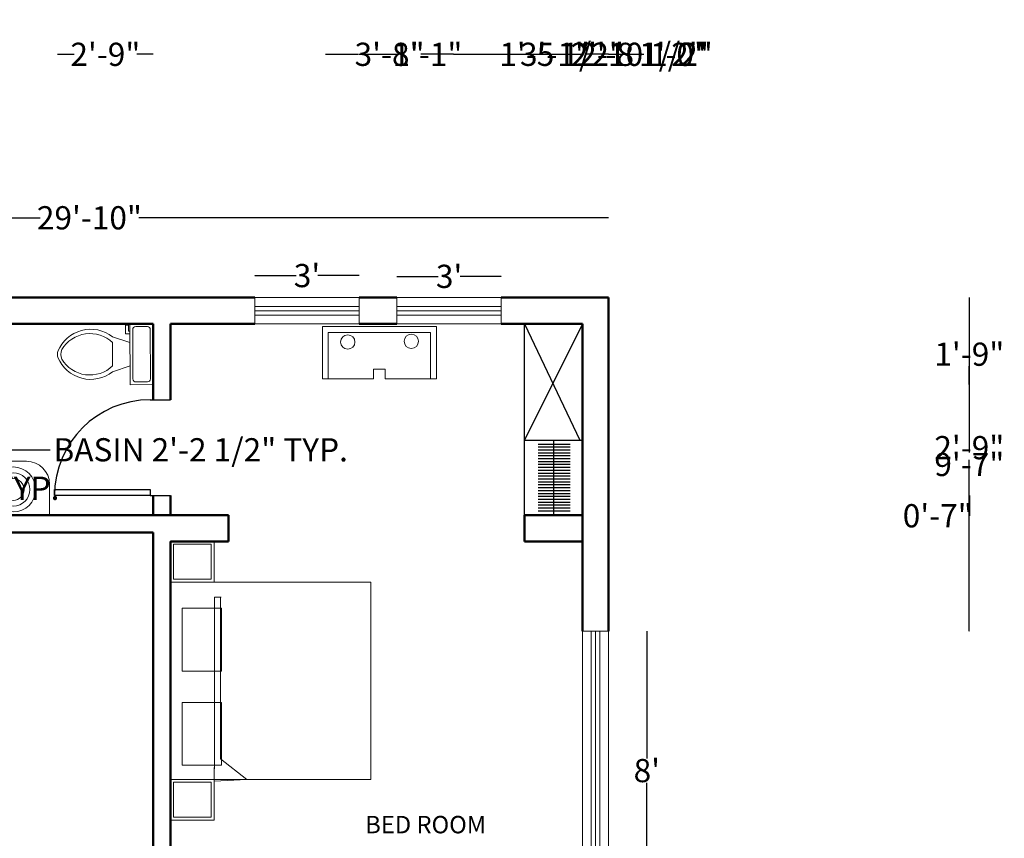
# Model space of a CAD drawing. Units: inches. Extents: x -135167 to -134597, y 156853 to 157819.
# Tile 5 of 5: x -134948 to -134608, y 157537 to 157819. Entities that reach past the tile are written whole.
import ezdxf

# ---------------------------------------------------------------- set-up
doc = ezdxf.new("R2010")
doc.units = ezdxf.units.IN
doc.header["$MEASUREMENT"] = 0
for name, color, linetype, lineweight in [('A-ANNO-DIMS', 4, 'Continuous', 18), ('A-AREA-IDEN', 76, 'Continuous', 25), ('A-FLOR-CASE', 1, 'Continuous', 25), ('A-FLOR-FIXT', 3, 'Continuous', 20), ('A-FURN', 1, 'Continuous', 18), ('doors', 5, 'Continuous', 25), ('walls', 2, 'Continuous', 50), ('window', 6, 'Continuous', 18)]:
    doc.layers.add(name, color=color, linetype=linetype, lineweight=lineweight)
doc.styles.get("Standard").update_dxf_attribs({"font": 'arial.ttf'})
doc.dimstyles.get("Standard").update_dxf_attribs({"dimtxt": 8, "dimasz": 0.18, "dimexe": 0.18, "dimexo": 0.0625, "dimgap": 0.09, "dimtad": 0, "dimtih": 1, "dimtoh": 1, "dimdec": 0, "dimzin": 0, "dimdsep": 46, "dimlunit": 3, "dimtxsty": 'Standard', "dimblk": 'ARCHTICK', "dimcen": 0.09, "dimse1": 1, "dimse2": 1, "dimadec": 0, "dimazin": 0, "dimtfac": 1, "dimtdec": 0, "dimtofl": 0, "dimtmove": 0, "dimatfit": 3, "dimldrblk": 'DOTSMALL', "dimfxl": 1, "dimtolj": 1, "dimtzin": 0, "dimarcsym": 0})

# ---------------------------------------------------------------- blocks, each defined once
blk = doc.blocks.new('*U8')
for p, q in [((0, 0), (0, -6)), ((28, 0), (28, -6))]:
    blk.add_line(p, q)
blk.add_lwpolyline([(0, 0), (0, 28), (1.75, 28), (1.75, 0)], close=True)
blk.add_arc((0, 0), 28, 0, 90)
blk = doc.blocks.new('*U16')
for p, q in [((-9.51, 6.98), (-9.52, 9.98)), ((-9.52, 9.98), (-8.52, 9.98)), ((-8.01, 6.98), (-9.51, 6.98)), ((-8.52, 9.98), (-8.52, 7.98)), ((-8.52, 7.98), (-8.02, 7.98)), ((-8.01, 3.98), (-14.01, 5.97)), ((-13.99, -4.03), (-14.01, 3.97)), ((-7.99, -4.02), (-13.99, -6.03)), ((-5.98, -9.51), (-1.98, -9.5))]:
    blk.add_line(p, q)
blk.add_lwpolyline([(-7.98, -10.51), (0.02, -10.5), (-0.02, 10.5), (-8.02, 10.48)], close=True)
for points in [[(-7.02, 8.49), (-6.98, -8.51)], [(-2.02, 9.5), (-6.02, 9.49)], [(-0.98, -8.5), (-1.02, 8.5)]]:
    blk.add_lwpolyline(points)
for centre, radius, start, end in [((-21.57, -3.56), 12.17, 51.5766, 158.079), ((-21.81, -4.24), 11.33, 46.4753, 149.0544), ((-6.14, 8.61), 0.884, 81.9774, 188.2376), ((-1.89, 8.62), 0.884, 351.9774, 98.2376), ((-29, -0.05), 4, 164.9681, 195.247), ((-27.88, -0.05), 4, 155.8394, 204.3757), ((-21.59, 3.48), 12.17, 202.136, 308.6382), ((-21.83, 4.16), 11.33, 211.1605, 313.7396), ((-6.11, -8.64), 0.884, 171.9774, 278.2376), ((-1.86, -8.63), 0.884, 261.9774, 8.2376)]:
    blk.add_arc(centre, radius, start, end)
blk = doc.blocks.new('_ArchTick')
at = {"color": 0, "linetype": 'ByBlock', "const_width": 0.15}
blk.add_lwpolyline([(-0.5, -0.5), (0.5, 0.5)], dxfattribs=at)
blk = doc.blocks.new('*D19')
at = {"layer": 'A-ANNO-DIMS', "color": 0, "lineweight": -2, "transparency": 16777216}
for p, q in [((-135102.89, 157750.46), (-134940.89, 157750.46)), ((-134744.89, 157750.46), (-134906.88, 157750.46))]:
    blk.add_line(p, q, dxfattribs=at)
at = {"layer": 'Defpoints', "color": 0, "transparency": 16777216}
for p in [(-134744.89, 157750.46), (-135102.89, 157722.94), (-134744.89, 157722.94)]:
    blk.add_point(p, dxfattribs=at)
at = {"layer": 'A-ANNO-DIMS', "color": 0, "lineweight": -2, "transparency": 16777216, "xscale": 0.18, "yscale": 0.18, "zscale": 0.18, "rotation": 180}
blk.add_blockref('_ArchTick', (-135102.89, 157750.46), dxfattribs=at)
at = {"layer": 'A-ANNO-DIMS', "color": 0, "lineweight": -2, "transparency": 16777216, "xscale": 0.18, "yscale": 0.18, "zscale": 0.18}
blk.add_blockref('_ArchTick', (-134744.89, 157750.46), dxfattribs=at)
at = {"layer": 'A-ANNO-DIMS', "color": 0, "transparency": 16777216, "insert": (-134923.89, 157750.46), "char_height": 8, "attachment_point": 5}
blk.add_mtext('\\A1;29\'-10"', dxfattribs=at)
blk = doc.blocks.new('_DotSmall')
at = {"color": 0, "linetype": 'ByBlock', "const_width": 0.5}
blk.add_lwpolyline([(-0.0625, 0, 1), (0.0625, 0, 1)], format="xyb", close=True, dxfattribs=at)
blk = doc.blocks.new('*D28')
at = {"layer": 'A-ANNO-DIMS', "color": 0, "lineweight": -2, "transparency": 16777216}
for p, q in [((-134731.73, 157607.94), (-134731.73, 157564.12)), ((-134731.73, 157511.94), (-134731.73, 157555.77))]:
    blk.add_line(p, q, dxfattribs=at)
at = {"layer": 'Defpoints', "color": 0, "transparency": 16777216}
for p in [(-134744.89, 157607.94), (-134731.73, 157607.94), (-134744.89, 157511.94)]:
    blk.add_point(p, dxfattribs=at)
at = {"layer": 'A-ANNO-DIMS', "color": 0, "lineweight": -2, "transparency": 16777216, "xscale": 0.18, "yscale": 0.18, "zscale": 0.18}
for p, rotation in [((-134731.73, 157607.94), 90), ((-134731.73, 157511.94), 270)]:
    blk.add_blockref('_ArchTick', p, dxfattribs=dict(at, rotation=rotation))
at = {"layer": 'A-ANNO-DIMS', "color": 0, "transparency": 16777216, "insert": (-134731.73, 157559.94), "char_height": 8, "attachment_point": 5}
blk.add_mtext("\\A1;8'", dxfattribs=at)
blk = doc.blocks.new('*D29')
at = {"layer": 'A-ANNO-DIMS', "color": 0, "lineweight": -2, "transparency": 16777216}
for p, q in [((-134817.89, 157730.27), (-134803.65, 157730.27)), ((-134781.89, 157730.27), (-134796.12, 157730.27))]:
    blk.add_line(p, q, dxfattribs=at)
at = {"layer": 'Defpoints', "color": 0, "transparency": 16777216}
for p in [(-134817.89, 157730.27), (-134817.89, 157722.94), (-134781.89, 157722.94)]:
    blk.add_point(p, dxfattribs=at)
at = {"layer": 'A-ANNO-DIMS', "color": 0, "lineweight": -2, "transparency": 16777216, "xscale": 0.18, "yscale": 0.18, "zscale": 0.18, "rotation": 180}
blk.add_blockref('_ArchTick', (-134817.89, 157730.27), dxfattribs=at)
at = {"layer": 'A-ANNO-DIMS', "color": 0, "lineweight": -2, "transparency": 16777216, "xscale": 0.18, "yscale": 0.18, "zscale": 0.18}
blk.add_blockref('_ArchTick', (-134781.89, 157730.27), dxfattribs=at)
at = {"layer": 'A-ANNO-DIMS', "color": 0, "transparency": 16777216, "insert": (-134799.89, 157730.27), "char_height": 8, "attachment_point": 5}
blk.add_mtext("\\A1;3'", dxfattribs=at)
blk = doc.blocks.new('*D30')
at = {"layer": 'A-ANNO-DIMS', "color": 0, "lineweight": -2, "transparency": 16777216}
for p, q in [((-134866.89, 157730.54), (-134852.65, 157730.54)), ((-134830.89, 157730.54), (-134845.12, 157730.54))]:
    blk.add_line(p, q, dxfattribs=at)
at = {"layer": 'Defpoints', "color": 0, "transparency": 16777216}
for p in [(-134866.89, 157730.54), (-134866.89, 157722.94), (-134830.89, 157722.94)]:
    blk.add_point(p, dxfattribs=at)
at = {"layer": 'A-ANNO-DIMS', "color": 0, "lineweight": -2, "transparency": 16777216, "xscale": 0.18, "yscale": 0.18, "zscale": 0.18, "rotation": 180}
blk.add_blockref('_ArchTick', (-134866.89, 157730.54), dxfattribs=at)
at = {"layer": 'A-ANNO-DIMS', "color": 0, "lineweight": -2, "transparency": 16777216, "xscale": 0.18, "yscale": 0.18, "zscale": 0.18}
blk.add_blockref('_ArchTick', (-134830.89, 157730.54), dxfattribs=at)
at = {"layer": 'A-ANNO-DIMS', "color": 0, "transparency": 16777216, "insert": (-134848.89, 157730.54), "char_height": 8, "attachment_point": 5}
blk.add_mtext("\\A1;3'", dxfattribs=at)
blk = doc.blocks.new('BED-DOUBLE-WITH-NIGHTSTANDS')
for p, q in [((0, 82.04), (69, 82.04)), ((69, 82.04), (69, 14.04)), ((15.15, 17.72), (15.15, 76.81)), ((15.15, 76.81), (17.47, 76.81)), ((17.23, 76.81), (17.23, 21.1)), ((17.23, 21.1), (26.3, 14.04)), ((15.01, 13.43), (15.01, 18.09)), ((69, 14.04), (0, 14.04)), ((26.3, 14.04), (15.01, 13.43))]:
    blk.add_line(p, q)
for points in [[(0, 96.09), (15.01, 96.09), (15.01, 82.04), (0, 82.04)], [(1, 95.09), (14.01, 95.09), (14.01, 83.04), (1, 83.04)], [(3.95, 51.37), (17.49, 51.37), (17.49, 73.01), (3.95, 73.01)], [(3.95, 18.92), (17.49, 18.92), (17.49, 40.56), (3.95, 40.56)], [(0, 14.04), (15.01, 14.04), (15.01, 0), (0, 0)], [(1, 13.04), (14.01, 13.04), (14.01, 1), (1, 1)]]:
    blk.add_lwpolyline(points, close=True)
blk = doc.blocks.new('BASIN-WALL')
for points in [[(18.54, 18.59), (7.9, 18.59)], [(0, 10.69), (0, 0)], [(26.44, 0), (26.44, 10.69)]]:
    blk.add_lwpolyline(points)
for radius in [7.75, 5.75, 3.75]:
    blk.add_circle((13.93, 8.88), radius)
for centre, start, end in [((7.9, 10.69), 90, 180), ((18.54, 10.69), 0, 90)]:
    blk.add_arc(centre, 7.9, start, end)
blk = doc.blocks.new('WIN-36IN')
for p, q in [((0, 0), (0, 9)), ((0, 9), (36, 9)), ((36, 0), (36, 9)), ((0, 6), (36, 6)), ((0, 4.5), (36, 4.5)), ((0, 3), (36, 3)), ((0, 0), (36, 0))]:
    blk.add_line(p, q)
blk = doc.blocks.new('WIN-96IN')
for p, q in [((0, 96), (9, 96)), ((0, 96), (0, 0)), ((3, 96), (3, 0)), ((4.5, 96), (4.5, 0)), ((6, 96), (6, 0)), ((9, 96), (9, 0)), ((0, 0), (9, 0))]:
    blk.add_line(p, q)
blk = doc.blocks.new('*D52')
at = {"layer": 'A-ANNO-DIMS', "color": 0, "lineweight": -2, "transparency": 16777216}
for p, q in [((-134964.09, 157670.5), (-134937.65, 157670.5)), ((-134937.65, 157670.5), (-134937.47, 157670.5))]:
    blk.add_line(p, q, dxfattribs=at)
at = {"layer": 'Defpoints', "color": 0, "transparency": 16777216}
for p in [(-134937.65, 157670.5), (-134964.09, 157666.53), (-134937.65, 157666.53)]:
    blk.add_point(p, dxfattribs=at)
at = {"layer": 'A-ANNO-DIMS', "color": 0, "lineweight": -2, "transparency": 16777216, "xscale": 0.18, "yscale": 0.18, "zscale": 0.18, "rotation": 180}
blk.add_blockref('_ArchTick', (-134964.09, 157670.5), dxfattribs=at)
at = {"layer": 'A-ANNO-DIMS', "color": 0, "lineweight": -2, "transparency": 16777216, "xscale": 0.18, "yscale": 0.18, "zscale": 0.18}
blk.add_blockref('_ArchTick', (-134937.65, 157670.5), dxfattribs=at)
at = {"layer": 'A-ANNO-DIMS', "color": 0, "transparency": 16777216, "insert": (-134885.53, 157670.5), "char_height": 8, "attachment_point": 5}
blk.add_mtext('\\A1;BASIN 2\'-2 1/2" TYP.', dxfattribs=at)
blk = doc.blocks.new('*D53')
at = {"layer": 'A-ANNO-DIMS', "color": 0, "lineweight": -2, "transparency": 16777216}
for p, q in [((-134968.06, 157666.53), (-134968.06, 157661.46)), ((-134968.06, 157647.94), (-134968.06, 157653.01))]:
    blk.add_line(p, q, dxfattribs=at)
at = {"layer": 'Defpoints', "color": 0, "transparency": 16777216}
for p in [(-134968.06, 157666.53), (-134964.09, 157666.53), (-134964.09, 157647.94)]:
    blk.add_point(p, dxfattribs=at)
at = {"layer": 'A-ANNO-DIMS', "color": 0, "lineweight": -2, "transparency": 16777216, "xscale": 0.18, "yscale": 0.18, "zscale": 0.18}
for p, rotation in [((-134968.06, 157666.53), 90), ((-134968.06, 157647.94), 270)]:
    blk.add_blockref('_ArchTick', p, dxfattribs=dict(at, rotation=rotation))
at = {"layer": 'A-ANNO-DIMS', "color": 0, "transparency": 16777216, "insert": (-134968.06, 157657.24), "char_height": 8, "attachment_point": 5}
blk.add_mtext('\\A1;1\'-6 1/2" TYP.', dxfattribs=at)
blk = doc.blocks.new('*D61')
at = {"layer": 'A-ANNO-DIMS', "color": 0, "lineweight": -2, "transparency": 16777216}
for p, q in [((-134620.54, 157722.94), (-134620.54, 157669.62)), ((-134620.54, 157607.94), (-134620.54, 157661.27))]:
    blk.add_line(p, q, dxfattribs=at)
at = {"layer": 'Defpoints', "color": 0, "transparency": 16777216}
for p in [(-134744.89, 157722.94), (-134744.89, 157607.94), (-134620.54, 157607.94)]:
    blk.add_point(p, dxfattribs=at)
at = {"layer": 'A-ANNO-DIMS', "color": 0, "lineweight": -2, "transparency": 16777216, "xscale": 0.18, "yscale": 0.18, "zscale": 0.18}
for p, rotation in [((-134620.54, 157722.94), 90), ((-134620.54, 157607.94), 270)]:
    blk.add_blockref('_ArchTick', p, dxfattribs=dict(at, rotation=rotation))
at = {"layer": 'A-ANNO-DIMS', "color": 0, "transparency": 16777216, "insert": (-134620.54, 157665.44), "char_height": 8, "attachment_point": 5}
blk.add_mtext('\\A1;9\'-7"', dxfattribs=at)
blk = doc.blocks.new('*D67')
at = {"layer": 'A-ANNO-DIMS', "color": 0, "lineweight": -2, "transparency": 16777216}
for p, q in [((-134744.89, 157806.8), (-134732.89, 157806.8)), ((-134732.89, 157806.8), (-134732.71, 157806.8))]:
    blk.add_line(p, q, dxfattribs=at)
at = {"layer": 'Defpoints', "color": 0, "transparency": 16777216}
for p in [(-134732.89, 157806.8), (-134744.89, 157145.8), (-134732.89, 157145.8)]:
    blk.add_point(p, dxfattribs=at)
at = {"layer": 'A-ANNO-DIMS', "color": 0, "lineweight": -2, "transparency": 16777216, "xscale": 0.18, "yscale": 0.18, "zscale": 0.18, "rotation": 180}
blk.add_blockref('_ArchTick', (-134744.89, 157806.8), dxfattribs=at)
at = {"layer": 'A-ANNO-DIMS', "color": 0, "lineweight": -2, "transparency": 16777216, "xscale": 0.18, "yscale": 0.18, "zscale": 0.18}
blk.add_blockref('_ArchTick', (-134732.89, 157806.8), dxfattribs=at)
at = {"layer": 'A-ANNO-DIMS', "color": 0, "transparency": 16777216, "insert": (-134722.36, 157806.8), "char_height": 8, "attachment_point": 5}
blk.add_mtext('\\A1;1\'-0"', dxfattribs=at)
blk = doc.blocks.new('*D70')
at = {"layer": 'A-ANNO-DIMS', "color": 0, "lineweight": -2, "transparency": 16777216}
for p, q in [((-134781.89, 157806.8), (-134774.11, 157806.8)), ((-134744.89, 157806.8), (-134752.67, 157806.8))]:
    blk.add_line(p, q, dxfattribs=at)
at = {"layer": 'Defpoints', "color": 0, "transparency": 16777216}
for p in [(-134744.89, 157806.8), (-134781.89, 157722.94), (-134744.89, 157722.94)]:
    blk.add_point(p, dxfattribs=at)
at = {"layer": 'A-ANNO-DIMS', "color": 0, "lineweight": -2, "transparency": 16777216, "xscale": 0.18, "yscale": 0.18, "zscale": 0.18, "rotation": 180}
blk.add_blockref('_ArchTick', (-134781.89, 157806.8), dxfattribs=at)
at = {"layer": 'A-ANNO-DIMS', "color": 0, "lineweight": -2, "transparency": 16777216, "xscale": 0.18, "yscale": 0.18, "zscale": 0.18}
blk.add_blockref('_ArchTick', (-134744.89, 157806.8), dxfattribs=at)
at = {"layer": 'A-ANNO-DIMS', "color": 0, "transparency": 16777216, "insert": (-134763.39, 157806.8), "char_height": 8, "attachment_point": 5}
blk.add_mtext('\\A1;3\'-1"', dxfattribs=at)
blk = doc.blocks.new('*D71')
at = {"layer": 'A-ANNO-DIMS', "color": 0, "lineweight": -2, "transparency": 16777216}
for p, q in [((-134830.89, 157806.8), (-134817.89, 157806.8)), ((-134817.89, 157806.8), (-134817.71, 157806.8))]:
    blk.add_line(p, q, dxfattribs=at)
at = {"layer": 'Defpoints', "color": 0, "transparency": 16777216}
for p in [(-134817.89, 157806.8), (-134830.89, 157722.94), (-134817.89, 157722.94)]:
    blk.add_point(p, dxfattribs=at)
at = {"layer": 'A-ANNO-DIMS', "color": 0, "lineweight": -2, "transparency": 16777216, "xscale": 0.18, "yscale": 0.18, "zscale": 0.18, "rotation": 180}
blk.add_blockref('_ArchTick', (-134830.89, 157806.8), dxfattribs=at)
at = {"layer": 'A-ANNO-DIMS', "color": 0, "lineweight": -2, "transparency": 16777216, "xscale": 0.18, "yscale": 0.18, "zscale": 0.18}
blk.add_blockref('_ArchTick', (-134817.89, 157806.8), dxfattribs=at)
at = {"layer": 'A-ANNO-DIMS', "color": 0, "transparency": 16777216, "insert": (-134807.36, 157806.8), "char_height": 8, "attachment_point": 5}
blk.add_mtext('\\A1;1\'-1"', dxfattribs=at)
blk = doc.blocks.new('*D73')
at = {"layer": 'A-ANNO-DIMS', "color": 0, "lineweight": -2, "transparency": 16777216}
for p, q in [((-134842.49, 157806.8), (-134831.13, 157806.8)), ((-134798.32, 157806.8), (-134809.69, 157806.8))]:
    blk.add_line(p, q, dxfattribs=at)
at = {"layer": 'Defpoints', "color": 0, "transparency": 16777216}
for p in [(-134798.32, 157806.8), (-134842.49, 157420.8), (-134798.32, 157420.8)]:
    blk.add_point(p, dxfattribs=at)
at = {"layer": 'A-ANNO-DIMS', "color": 0, "lineweight": -2, "transparency": 16777216, "xscale": 0.18, "yscale": 0.18, "zscale": 0.18, "rotation": 180}
blk.add_blockref('_ArchTick', (-134842.49, 157806.8), dxfattribs=at)
at = {"layer": 'A-ANNO-DIMS', "color": 0, "lineweight": -2, "transparency": 16777216, "xscale": 0.18, "yscale": 0.18, "zscale": 0.18}
blk.add_blockref('_ArchTick', (-134798.32, 157806.8), dxfattribs=at)
at = {"layer": 'A-ANNO-DIMS', "color": 0, "transparency": 16777216, "insert": (-134820.41, 157806.8), "char_height": 8, "attachment_point": 5}
blk.add_mtext('\\A1;3\'-8"', dxfattribs=at)
blk = doc.blocks.new('*D76')
at = {"layer": 'A-ANNO-DIMS', "color": 0, "lineweight": -2, "transparency": 16777216}
for p, q in [((-134786.25, 157806.8), (-134753.89, 157806.8)), ((-134753.89, 157806.8), (-134753.71, 157806.8))]:
    blk.add_line(p, q, dxfattribs=at)
at = {"layer": 'Defpoints', "color": 0, "transparency": 16777216}
for p in [(-134753.89, 157806.8), (-134753.89, 157473.94), (-134786.25, 157464.74)]:
    blk.add_point(p, dxfattribs=at)
at = {"layer": 'A-ANNO-DIMS', "color": 0, "lineweight": -2, "transparency": 16777216, "xscale": 0.18, "yscale": 0.18, "zscale": 0.18, "rotation": 180}
blk.add_blockref('_ArchTick', (-134786.25, 157806.8), dxfattribs=at)
at = {"layer": 'A-ANNO-DIMS', "color": 0, "lineweight": -2, "transparency": 16777216, "xscale": 0.18, "yscale": 0.18, "zscale": 0.18}
blk.add_blockref('_ArchTick', (-134753.89, 157806.8), dxfattribs=at)
at = {"layer": 'A-ANNO-DIMS', "color": 0, "transparency": 16777216, "insert": (-134733.59, 157806.8), "char_height": 8, "attachment_point": 5}
blk.add_mtext('\\A1;2\'-8 1/2"', dxfattribs=at)
blk = doc.blocks.new('*D77')
at = {"layer": 'A-ANNO-DIMS', "color": 0, "lineweight": -2, "transparency": 16777216}
for p, q in [((-134798.32, 157806.8), (-134780.93, 157806.8)), ((-134780.93, 157806.8), (-134780.75, 157806.8))]:
    blk.add_line(p, q, dxfattribs=at)
at = {"layer": 'Defpoints', "color": 0, "transparency": 16777216}
for p in [(-134780.93, 157806.8), (-134798.32, 157322.23), (-134780.93, 157308.36)]:
    blk.add_point(p, dxfattribs=at)
at = {"layer": 'A-ANNO-DIMS', "color": 0, "lineweight": -2, "transparency": 16777216, "xscale": 0.18, "yscale": 0.18, "zscale": 0.18, "rotation": 180}
blk.add_blockref('_ArchTick', (-134798.32, 157806.8), dxfattribs=at)
at = {"layer": 'A-ANNO-DIMS', "color": 0, "lineweight": -2, "transparency": 16777216, "xscale": 0.18, "yscale": 0.18, "zscale": 0.18}
blk.add_blockref('_ArchTick', (-134780.93, 157806.8), dxfattribs=at)
at = {"layer": 'A-ANNO-DIMS', "color": 0, "transparency": 16777216, "insert": (-134761.09, 157806.8), "char_height": 8, "attachment_point": 5}
blk.add_mtext('\\A1;1\'-5 1/2"', dxfattribs=at)
blk = doc.blocks.new('*D89')
at = {"layer": 'A-ANNO-DIMS', "color": 0, "lineweight": -2, "transparency": 16777216}
for p, q in [((-134620.54, 157687.72), (-134620.54, 157675.41)), ((-134620.54, 157654.75), (-134620.54, 157667.06))]:
    blk.add_line(p, q, dxfattribs=at)
at = {"layer": 'Defpoints', "color": 0, "transparency": 16777216}
for p in [(-134895.89, 157687.72), (-134620.54, 157687.72), (-134895.89, 157654.75)]:
    blk.add_point(p, dxfattribs=at)
at = {"layer": 'A-ANNO-DIMS', "color": 0, "lineweight": -2, "transparency": 16777216, "xscale": 0.18, "yscale": 0.18, "zscale": 0.18}
for p, rotation in [((-134620.54, 157687.72), 90), ((-134620.54, 157654.75), 270)]:
    blk.add_blockref('_ArchTick', p, dxfattribs=dict(at, rotation=rotation))
at = {"layer": 'A-ANNO-DIMS', "color": 0, "transparency": 16777216, "insert": (-134620.54, 157671.24), "char_height": 8, "attachment_point": 5}
blk.add_mtext('\\A1;2\'-9"', dxfattribs=at)
blk = doc.blocks.new('*D90')
at = {"layer": 'A-ANNO-DIMS', "color": 0, "lineweight": -2, "transparency": 16777216}
for p, q in [((-134791.39, 157806.8), (-134756.89, 157806.8)), ((-134756.89, 157806.8), (-134756.71, 157806.8))]:
    blk.add_line(p, q, dxfattribs=at)
at = {"layer": 'Defpoints', "color": 0, "transparency": 16777216}
for p in [(-134756.89, 157806.8), (-134791.39, 156969.8), (-134756.89, 156969.8)]:
    blk.add_point(p, dxfattribs=at)
at = {"layer": 'A-ANNO-DIMS', "color": 0, "lineweight": -2, "transparency": 16777216, "xscale": 0.18, "yscale": 0.18, "zscale": 0.18, "rotation": 180}
blk.add_blockref('_ArchTick', (-134791.39, 157806.8), dxfattribs=at)
at = {"layer": 'A-ANNO-DIMS', "color": 0, "lineweight": -2, "transparency": 16777216, "xscale": 0.18, "yscale": 0.18, "zscale": 0.18}
blk.add_blockref('_ArchTick', (-134756.89, 157806.8), dxfattribs=at)
at = {"layer": 'A-ANNO-DIMS', "color": 0, "transparency": 16777216, "insert": (-134733.49, 157806.8), "char_height": 8, "attachment_point": 5}
blk.add_mtext('\\A1;2\'-10 1/2"', dxfattribs=at)
blk = doc.blocks.new('*D92')
at = {"layer": 'A-ANNO-DIMS', "color": 0, "lineweight": -2, "transparency": 16777216}
for p, q in [((-134987.89, 156858.2), (-134955.58, 156858.2)), ((-134901.89, 156858.2), (-134934.2, 156858.2))]:
    blk.add_line(p, q, dxfattribs=at)
at = {"layer": 'Defpoints', "color": 0, "transparency": 16777216}
for p in [(-134987.89, 157647.94), (-134901.89, 157647.94), (-134901.89, 156858.2)]:
    blk.add_point(p, dxfattribs=at)
at = {"layer": 'A-ANNO-DIMS', "color": 0, "lineweight": -2, "transparency": 16777216, "xscale": 0.18, "yscale": 0.18, "zscale": 0.18, "rotation": 180}
blk.add_blockref('_ArchTick', (-134987.89, 156858.2), dxfattribs=at)
at = {"layer": 'A-ANNO-DIMS', "color": 0, "lineweight": -2, "transparency": 16777216, "xscale": 0.18, "yscale": 0.18, "zscale": 0.18}
blk.add_blockref('_ArchTick', (-134901.89, 156858.2), dxfattribs=at)
at = {"layer": 'A-ANNO-DIMS', "color": 0, "transparency": 16777216, "insert": (-134944.89, 156858.2), "char_height": 8, "attachment_point": 5}
blk.add_mtext('\\A1;7\'-2"', dxfattribs=at)
blk = doc.blocks.new('*D95')
at = {"layer": 'A-ANNO-DIMS', "color": 0, "lineweight": -2, "transparency": 16777216}
for p, q in [((-134934.89, 157806.8), (-134929.18, 157806.8)), ((-134901.89, 157806.8), (-134907.59, 157806.8))]:
    blk.add_line(p, q, dxfattribs=at)
at = {"layer": 'Defpoints', "color": 0, "transparency": 16777216}
for p in [(-134901.89, 157806.8), (-134901.89, 157713.94), (-134934.89, 157703.39)]:
    blk.add_point(p, dxfattribs=at)
at = {"layer": 'A-ANNO-DIMS', "color": 0, "lineweight": -2, "transparency": 16777216, "xscale": 0.18, "yscale": 0.18, "zscale": 0.18, "rotation": 180}
blk.add_blockref('_ArchTick', (-134934.89, 157806.8), dxfattribs=at)
at = {"layer": 'A-ANNO-DIMS', "color": 0, "lineweight": -2, "transparency": 16777216, "xscale": 0.18, "yscale": 0.18, "zscale": 0.18}
blk.add_blockref('_ArchTick', (-134901.89, 157806.8), dxfattribs=at)
at = {"layer": 'A-ANNO-DIMS', "color": 0, "transparency": 16777216, "insert": (-134918.39, 157806.8), "char_height": 8, "attachment_point": 5}
blk.add_mtext('\\A1;2\'-9"', dxfattribs=at)
blk = doc.blocks.new('*D96')
at = {"layer": 'A-ANNO-DIMS', "color": 0, "lineweight": -2, "transparency": 16777216}
for p, q in [((-134620.54, 157713.94), (-134620.54, 157707.62)), ((-134620.54, 157692.95), (-134620.54, 157699.27))]:
    blk.add_line(p, q, dxfattribs=at)
at = {"layer": 'Defpoints', "color": 0, "transparency": 16777216}
for p in [(-134901.89, 157713.94), (-134901.87, 157692.95), (-134620.54, 157692.95)]:
    blk.add_point(p, dxfattribs=at)
at = {"layer": 'A-ANNO-DIMS', "color": 0, "lineweight": -2, "transparency": 16777216, "xscale": 0.18, "yscale": 0.18, "zscale": 0.18}
for p, rotation in [((-134620.54, 157713.94), 90), ((-134620.54, 157692.95), 270)]:
    blk.add_blockref('_ArchTick', p, dxfattribs=dict(at, rotation=rotation))
at = {"layer": 'A-ANNO-DIMS', "color": 0, "transparency": 16777216, "insert": (-134620.54, 157703.45), "char_height": 8, "attachment_point": 5}
blk.add_mtext('\\A1;1\'-9"', dxfattribs=at)
blk = doc.blocks.new('*D97')
at = {"layer": 'A-ANNO-DIMS', "color": 0, "lineweight": -2, "transparency": 16777216}
for p, q in [((-134620.535731, 157654.747874), (-134620.535731, 157647.942842)), ((-134620.535731, 157647.762842), (-134620.715731, 157647.762842)), ((-134620.535731, 157647.942842), (-134620.535731, 157647.762842))]:
    blk.add_line(p, q, dxfattribs=at)
at = {"layer": 'Defpoints', "color": 0, "transparency": 16777216}
for p in [(-134895.885731, 157654.747874), (-134901.885731, 157647.942842), (-134620.535731, 157647.942842)]:
    blk.add_point(p, dxfattribs=at)
at = {"layer": 'A-ANNO-DIMS', "color": 0, "lineweight": -2, "transparency": 16777216, "xscale": 0.18, "yscale": 0.18, "zscale": 0.18}
for p, rotation in [((-134620.535731, 157654.747874), 90), ((-134620.535731, 157647.942842), 270)]:
    blk.add_blockref('_ArchTick', p, dxfattribs=dict(at, rotation=rotation))
at = {"layer": 'A-ANNO-DIMS', "color": 0, "transparency": 16777216, "insert": (-134631.438746, 157647.762842), "char_height": 8, "attachment_point": 5}
blk.add_mtext('\\A1;0\'-7"', dxfattribs=at)

msp = doc.modelspace()

# ---------------------------------------------------------------- linework, layer by layer
at = {"layer": 'A-FLOR-CASE'}
for p, q in [((-134753.89, 157713.94), (-134773.89, 157713.94)), ((-134773.89, 157647.94), (-134773.89, 157713.94)), ((-134773.89, 157713.94), (-134754.82, 157673.79)), ((-134753.89, 157713.94), (-134773.89, 157673.79)), ((-134773.89, 157673.79), (-134753.89, 157673.79)), ((-134769.23, 157672.49), (-134758.11, 157672.49)), ((-134763.89, 157673.79), (-134763.89, 157647.94)), ((-134769.23, 157671.49), (-134758.11, 157671.49)), ((-134769.23, 157670.49), (-134758.11, 157670.49)), ((-134769.23, 157669.49), (-134758.11, 157669.49)), ((-134769.23, 157668.49), (-134758.11, 157668.49)), ((-134769.23, 157667.49), (-134758.11, 157667.49)), ((-134769.23, 157666.49), (-134758.11, 157666.49)), ((-134769.23, 157665.49), (-134758.11, 157665.49)), ((-134769.23, 157664.49), (-134758.11, 157664.49)), ((-134769.23, 157663.49), (-134758.11, 157663.49)), ((-134769.23, 157662.49), (-134758.11, 157662.49)), ((-134769.23, 157661.49), (-134758.11, 157661.49)), ((-134769.23, 157660.49), (-134758.11, 157660.49)), ((-134769.23, 157659.49), (-134758.11, 157659.49)), ((-134769.23, 157658.49), (-134758.11, 157658.49)), ((-134769.23, 157657.49), (-134758.11, 157657.49)), ((-134769.23, 157656.49), (-134758.11, 157656.49)), ((-134769.23, 157655.49), (-134758.11, 157655.49)), ((-134769.23, 157654.49), (-134758.11, 157654.49)), ((-134769.23, 157653.49), (-134758.11, 157653.49)), ((-134769.23, 157652.49), (-134758.11, 157652.49)), ((-134769.23, 157651.49), (-134758.11, 157651.49)), ((-134769.23, 157650.49), (-134758.11, 157650.49)), ((-134769.23, 157649.49), (-134758.11, 157649.49))]:
    msp.add_line(p, q, dxfattribs=at)
at = {"layer": 'A-FURN'}
for p, q in [((-134841.57, 157696.99), (-134841.57, 157694.99)), ((-134825.93, 157694.99), (-134825.93, 157698.23)), ((-134825.93, 157698.23), (-134821.93, 157698.23)), ((-134821.93, 157694.99), (-134821.93, 157698.23)), ((-134806.28, 157696.99), (-134806.28, 157694.99))]:
    msp.add_line(p, q, dxfattribs=at)
for points in [[(-134825.93, 157694.99), (-134843.57, 157694.99), (-134843.57, 157712.96), (-134804.28, 157712.96), (-134804.28, 157694.99), (-134821.93, 157694.99)], [(-134841.57, 157696.99), (-134841.57, 157710.96), (-134806.28, 157710.96), (-134806.28, 157696.99)]]:
    msp.add_lwpolyline(points, dxfattribs=at)
for centre in [(-134834.82, 157707.64), (-134812.91, 157707.88)]:
    msp.add_circle(centre, 2.47, dxfattribs=at)
at = {"layer": 'doors'}
for p, q in [((-134901.89, 157687.72), (-134895.89, 157687.72)), ((-134901.89, 157654.75), (-134895.89, 157654.75))]:
    msp.add_line(p, q, dxfattribs=at)
at = {"layer": 'walls'}
for p, q in [((-135102.89, 157722.94), (-134866.89, 157722.94)), ((-134830.89, 157722.94), (-134817.89, 157722.94)), ((-134781.89, 157722.94), (-134744.89, 157722.94)), ((-134744.89, 157607.94), (-134744.89, 157722.94)), ((-134987.89, 157713.94), (-134901.89, 157713.94)), ((-134901.89, 157687.72), (-134901.89, 157713.94)), ((-134895.89, 157713.94), (-134866.89, 157713.94)), ((-134895.89, 157687.72), (-134895.89, 157713.94)), ((-134830.89, 157713.94), (-134817.89, 157713.94)), ((-134781.89, 157713.94), (-134753.89, 157713.94)), ((-134753.89, 157607.94), (-134753.89, 157713.94)), ((-134901.89, 157647.94), (-134901.89, 157654.75)), ((-134895.89, 157647.94), (-134895.89, 157654.75)), ((-134987.89, 157647.94), (-134875.89, 157647.94)), ((-134875.89, 157638.94), (-134875.89, 157647.94)), ((-134773.89, 157638.94), (-134773.89, 157647.94)), ((-134773.89, 157647.94), (-134753.89, 157647.94)), ((-134993.89, 157641.94), (-134901.89, 157641.94)), ((-134901.89, 157480.94), (-134901.89, 157641.94)), ((-134895.89, 157480.94), (-134895.89, 157638.94)), ((-134895.89, 157638.94), (-134875.89, 157638.94)), ((-134773.89, 157638.94), (-134753.89, 157638.94))]:
    msp.add_line(p, q, dxfattribs=at)
at = {"layer": 'window'}
for p, q in [((-134866.89, 157713.94), (-134866.89, 157722.94)), ((-134866.89, 157722.94), (-134830.89, 157722.94)), ((-134830.89, 157716.94), (-134830.89, 157722.94)), ((-134866.89, 157719.94), (-134830.89, 157719.94)), ((-134866.89, 157718.44), (-134830.89, 157718.44)), ((-134866.89, 157716.94), (-134830.89, 157716.94)), ((-134830.89, 157713.94), (-134830.89, 157716.94)), ((-134866.89, 157713.94), (-134830.89, 157713.94))]:
    msp.add_line(p, q, dxfattribs=at)

# ---------------------------------------------------------------- block references
at = {"layer": 'A-FLOR-FIXT'}
for name, p in [('*U16', (-134901.89, 157703.45)), ('BASIN-WALL', (-134964.09, 157647.94))]:
    msp.add_blockref(name, p, dxfattribs=at)
at = {"layer": 'A-FURN'}
msp.add_blockref('BED-DOUBLE-WITH-NIGHTSTANDS', (-134895.89, 157542.86), dxfattribs=at)
at = {"layer": 'doors', "xscale": 1.177709194970221, "yscale": 1.177709194970221, "zscale": 1.177709194970221, "rotation": 90.00000000000003}
msp.add_blockref('*U8', (-134902.95, 157654.75), dxfattribs=at)
at = {"layer": 'window'}
for name, p in [('WIN-36IN', (-134817.89, 157713.94)), ('WIN-96IN', (-134753.89, 157511.94))]:
    msp.add_blockref(name, p, dxfattribs=at)

# ---------------------------------------------------------------- texts
at = {"layer": 'A-AREA-IDEN'}
msp.add_text('BED ROOM ', height=6, dxfattribs=at).set_placement((-134828.8, 157538.32))

# ---------------------------------------------------------------- dimensions: what is measured, and where the dimension line sits
at = {"layer": 'A-ANNO-DIMS'}
for base, p1, p2, override, picture, middle in [((-134780.93, 157806.8), (-134798.32, 157322.23), (-134780.93, 157308.36), {"dimdec": 1, "dimlfac": 1, "dimrnd": 0, "dimzin": 1, "dimdsep": 46, "dimlunit": 4, "dimfrac": 2}, '*D77', (-134761.09, 157806.8)), ((-134756.89, 157806.8), (-134791.39, 156969.8), (-134756.89, 156969.8), {"dimdec": 1, "dimlfac": 1, "dimrnd": 0, "dimzin": 1, "dimdsep": 46, "dimlunit": 4, "dimfrac": 2}, '*D90', (-134733.49, 157806.8)), ((-134753.89, 157806.8), (-134786.25, 157464.74), (-134753.89, 157473.94), {"dimdec": 1, "dimlfac": 1, "dimrnd": 0, "dimzin": 1, "dimdsep": 46, "dimlunit": 4, "dimfrac": 2}, '*D76', (-134733.59, 157806.8)), ((-134901.89, 157806.8), (-134934.89, 157703.39), (-134901.89, 157713.94), {"dimdec": 1, "dimlfac": 1, "dimrnd": 0, "dimzin": 1, "dimdsep": 46, "dimlunit": 4, "dimfrac": 2}, '*D95', (-134918.39, 157806.8)), ((-134798.32, 157806.8), (-134842.49, 157420.8), (-134798.32, 157420.8), {"dimdec": 1, "dimlfac": 1, "dimrnd": 0, "dimzin": 1, "dimdsep": 46, "dimlunit": 4, "dimfrac": 2}, '*D73', (-134820.41, 157806.8)), ((-134817.89, 157806.8), (-134830.89, 157722.94), (-134817.89, 157722.94), {"dimdec": 1, "dimlfac": 1, "dimrnd": 0, "dimzin": 1, "dimdsep": 46, "dimlunit": 4, "dimfrac": 2}, '*D71', (-134807.36, 157806.8)), ((-134744.89, 157806.8), (-134781.89, 157722.94), (-134744.89, 157722.94), {"dimdec": 1, "dimlfac": 1, "dimrnd": 0, "dimzin": 1, "dimdsep": 46, "dimlunit": 4, "dimfrac": 2}, '*D70', (-134763.39, 157806.8)), ((-134732.89, 157806.8), (-134744.89, 157145.8), (-134732.89, 157145.8), {"dimdec": 1, "dimlfac": 1, "dimrnd": 0, "dimzin": 1, "dimdsep": 46, "dimlunit": 4, "dimfrac": 2}, '*D67', (-134722.36, 157806.8)), ((-134744.89, 157750.46), (-135102.89, 157722.94), (-134744.89, 157722.94), {"dimclrd": 0, "dimclre": 0, "dimclrt": 0}, '*D19', (-134923.89, 157750.46)), ((-134866.89, 157730.54), (-134830.89, 157722.94), (-134866.89, 157722.94), {"dimclrd": 0, "dimclre": 0, "dimclrt": 0}, '*D30', (-134848.89, 157730.54)), ((-134817.89, 157730.27), (-134781.89, 157722.94), (-134817.89, 157722.94), {"dimclrd": 0, "dimclre": 0, "dimclrt": 0}, '*D29', (-134799.89, 157730.27)), ((-134901.89, 156858.2), (-134987.89, 157647.94), (-134901.89, 157647.94), {"dimdec": 1, "dimlfac": 1, "dimrnd": 0, "dimzin": 1, "dimdsep": 46, "dimlunit": 4, "dimfrac": 2}, '*D92', (-134944.89, 156858.2))]:
    dim = msp.add_linear_dim(base=base, p1=p1, p2=p2, dimstyle='Standard', override=override, dxfattribs=at)
    dim.commit()
    dim.dimension.update_dxf_attribs({"geometry": picture, "text_midpoint": middle})
for base, p1, p2, override, picture, middle in [((-134620.54, 157607.94), (-134744.89, 157722.94), (-134744.89, 157607.94), {"dimdec": 1, "dimlfac": 1, "dimrnd": 0, "dimzin": 1, "dimdsep": 46, "dimlunit": 4, "dimfrac": 2}, '*D61', (-134620.54, 157665.44)), ((-134620.54, 157692.95), (-134901.89, 157713.94), (-134901.87, 157692.95), {"dimdec": 1, "dimlfac": 1, "dimrnd": 0, "dimzin": 1, "dimdsep": 46, "dimlunit": 4, "dimfrac": 2}, '*D96', (-134620.54, 157703.45)), ((-134620.54, 157687.72), (-134895.89, 157654.75), (-134895.89, 157687.72), {"dimdec": 1, "dimlfac": 1, "dimrnd": 0, "dimzin": 1, "dimdsep": 46, "dimlunit": 4, "dimfrac": 2}, '*D89', (-134620.54, 157671.24)), ((-134620.54, 157647.94), (-134895.89, 157654.75), (-134901.89, 157647.94), {"dimdec": 1, "dimlfac": 1, "dimrnd": 0, "dimzin": 1, "dimdsep": 46, "dimlunit": 4, "dimfrac": 2}, '*D97', (-134631.44, 157647.76)), ((-134731.73, 157607.94), (-134744.89, 157511.94), (-134744.89, 157607.94), {"dimclrd": 0, "dimclre": 0, "dimclrt": 0}, '*D28', (-134731.73, 157559.94))]:
    dim = msp.add_linear_dim(base=base, p1=p1, p2=p2, angle=90, dimstyle='Standard', override=override, dxfattribs=at)
    dim.commit()
    dim.dimension.update_dxf_attribs({"geometry": picture, "text_midpoint": middle})
dim = msp.add_linear_dim(base=(-134937.65, 157670.5), p1=(-134964.09, 157666.53), p2=(-134937.65, 157666.53), text='BASIN <> TYP.', dimstyle='Standard', override={"dimdec": 1, "dimlfac": 1, "dimrnd": 0, "dimzin": 1, "dimdsep": 46, "dimlunit": 4, "dimfrac": 2}, dxfattribs=at)
dim.commit()
dim.dimension.update_dxf_attribs({"geometry": '*D52', "text_midpoint": (-134885.53, 157670.5)})
dim = msp.add_linear_dim(base=(-134968.06, 157666.53), p1=(-134964.09, 157647.94), p2=(-134964.09, 157666.53), angle=90, text='<> TYP.', dimstyle='Standard', override={"dimdec": 1, "dimlfac": 1, "dimrnd": 0, "dimzin": 1, "dimdsep": 46, "dimlunit": 4, "dimfrac": 2}, dxfattribs=at)
dim.commit()
dim.dimension.update_dxf_attribs({"geometry": '*D53', "text_midpoint": (-134968.06, 157657.24)})

doc.saveas('drawing.dxf')
